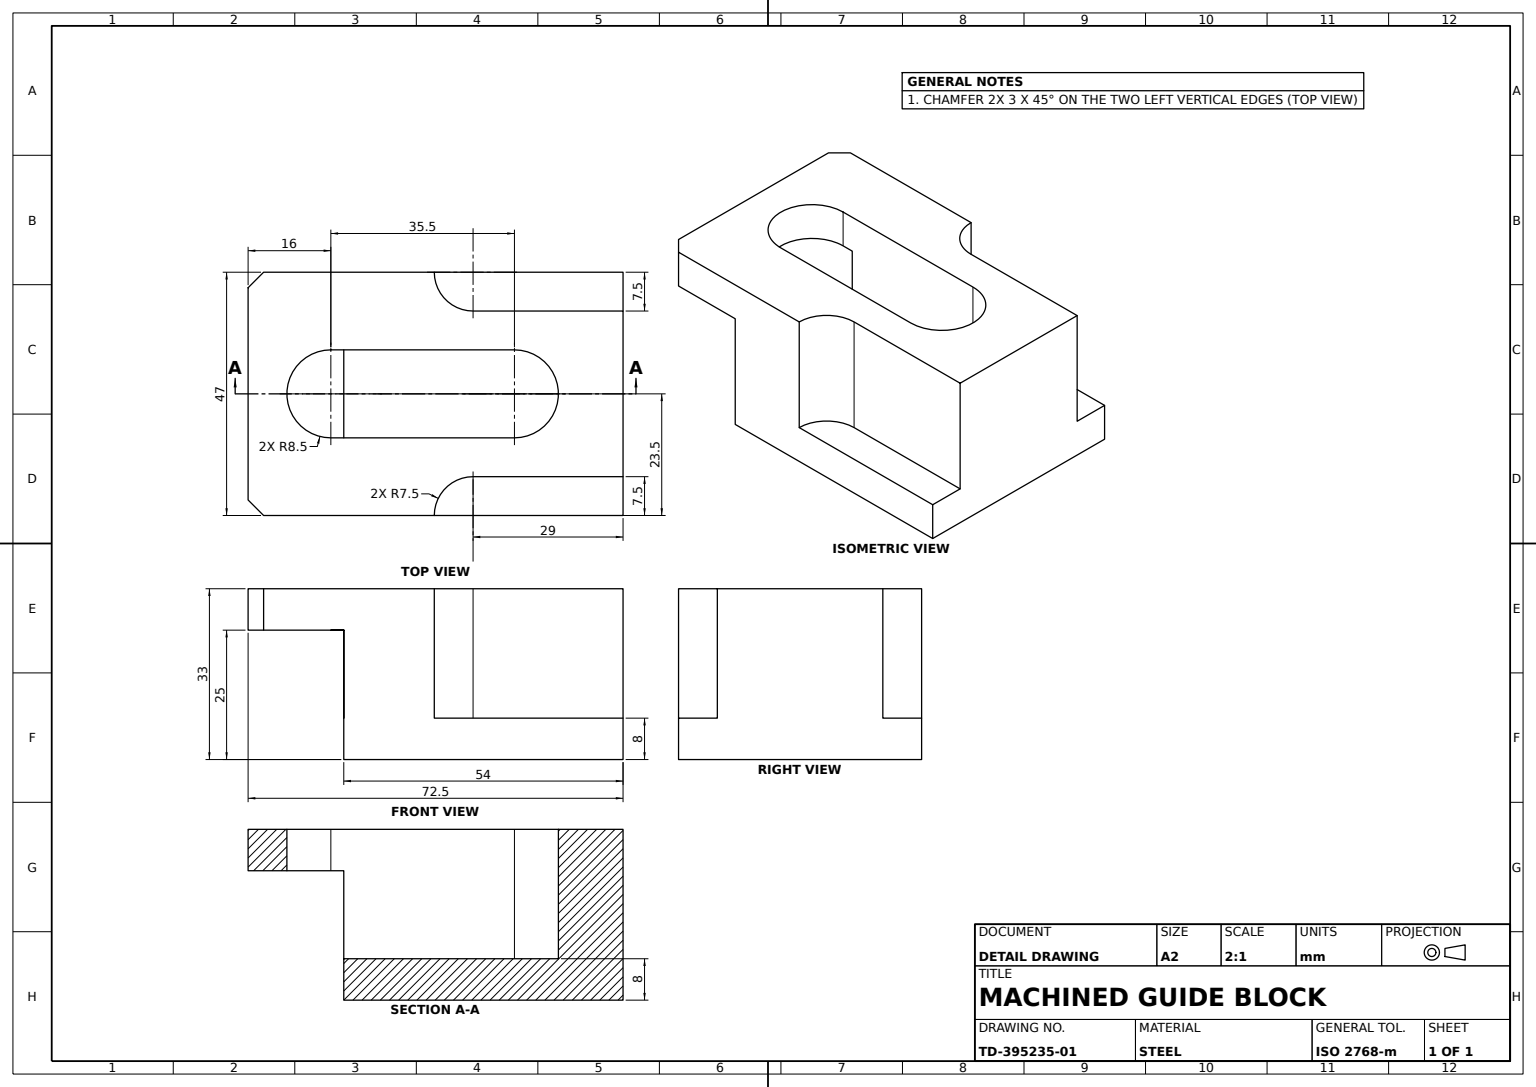
from build123d import *

# Parameters (mm, degrees)
BASE_BLOCK_DEPTH       = 47
SIDE_NOTCH_A_DEPTH     = 25
SIDE_NOTCH_B_DEPTH     = 25
GUIDE_SLOT_DEPTH       = 25
EDGE_CHAMFER_3X45_SIZE = 3


with BuildPart() as part:
    # Base Profile Sketch → Base Block (new body)
    with BuildSketch(Plane.XY):
        Polygon((0, 0), (54, 0), (54, 8), (54, 33), (-18.5, 33), (-18.5, 25), (0, 25), align=None)
    extrude(amount=-BASE_BLOCK_DEPTH)

    # Side Notch A Sketch → Side Notch A (cut)
    with BuildSketch(Plane(origin=(0, 33, 0), x_dir=(1, 0, 0), z_dir=(0, 1, 0))):
        with BuildLine():
            Line((54, 0), (54, 7.5))
            Line((54, 7.5), (25, 7.5))
            ThreePointArc((25, 7.5), (19.696699141, 5.303300859), (17.5, 0))
            Line((17.5, 0), (25, 0))
            Line((25, 0), (54, 0))
        make_face()
    extrude(amount=-SIDE_NOTCH_A_DEPTH, mode=Mode.SUBTRACT)

    # Side Notch B Sketch → Side Notch B (cut)
    with BuildSketch(Plane(origin=(0, 33, 0), x_dir=(1, 0, 0), z_dir=(0, 1, 0))):
        with BuildLine():
            Line((54, 47), (54, 39.5))
            Line((54, 39.5), (25, 39.5))
            ThreePointArc((25, 39.5), (19.696699141, 41.696699141), (17.5, 47))
            Line((17.5, 47), (25, 47))
            Line((25, 47), (54, 47))
        make_face()
    extrude(amount=-SIDE_NOTCH_B_DEPTH, mode=Mode.SUBTRACT)

    # Guide Slot Sketch → Guide Slot (cut)
    with BuildSketch(Plane(origin=(0, 33, 0), x_dir=(1, 0, 0), z_dir=(0, 1, 0))):
        with BuildLine():
            Line((-2.5, 32), (33, 32))
            ThreePointArc((33, 32), (41.5, 23.5), (33, 15))
            Line((33, 15), (-2.5, 15))
            ThreePointArc((-2.5, 15), (-11, 23.5), (-2.5, 32))
        make_face()
    extrude(amount=-GUIDE_SLOT_DEPTH, mode=Mode.SUBTRACT)

    # Edge Chamfer 3x45
    edge_chamfer_3x45_edges = [part.edges().sort_by_distance(p)[0] for p in [
        (-18.5, 29, -47),
        (-18.5, 29, 0),
    ]]
    chamfer(edge_chamfer_3x45_edges, length=EDGE_CHAMFER_3X45_SIZE)


solid = part.part
